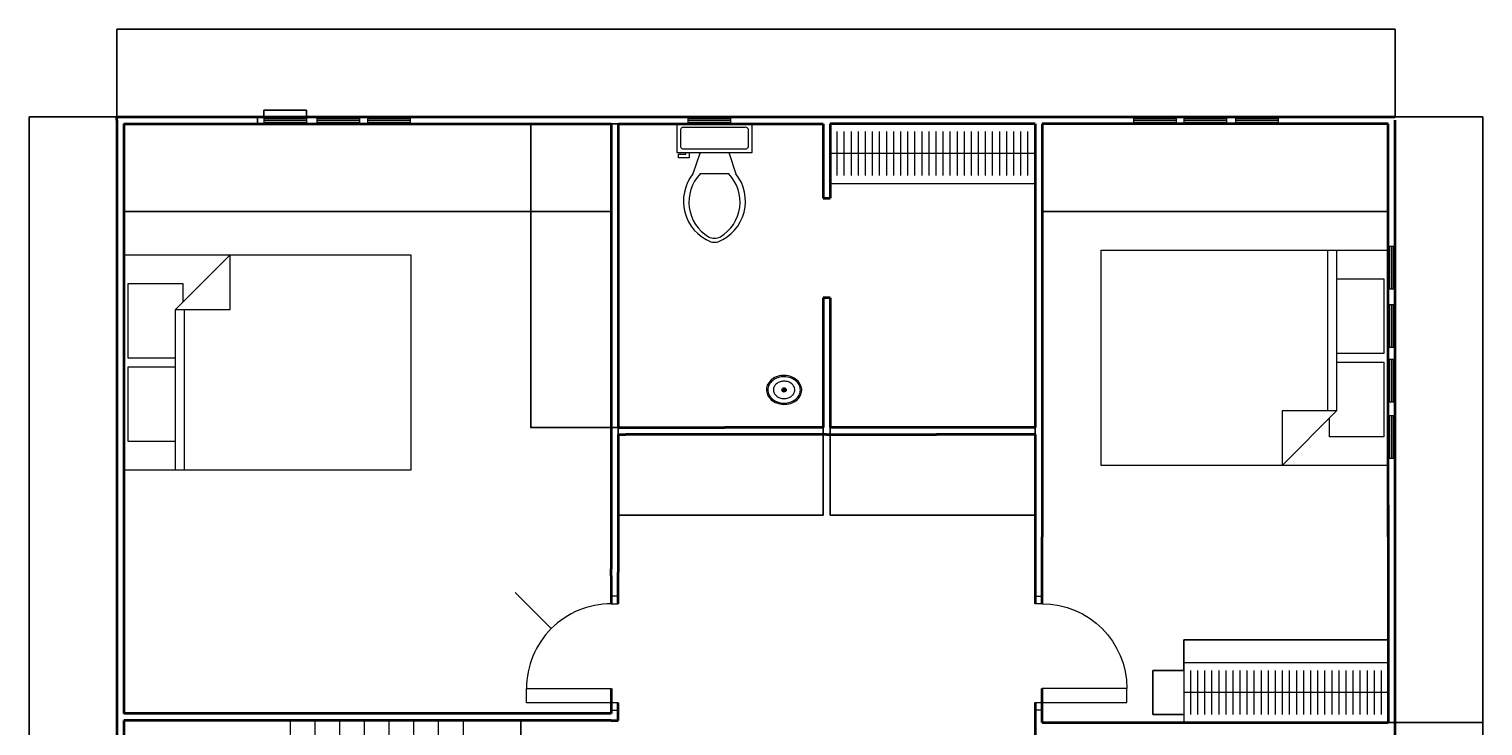
# Model space of a CAD drawing. Units: millimetres. Extents: x 1194 to 22780, y 83 to 13378.
# Tile 6 of 6: x 12489 to 22780, y 8443 to 13376. Entities that reach past the tile are written whole.
import ezdxf

# ---------------------------------------------------------------- set-up
doc = ezdxf.new("R2010")
doc.units = ezdxf.units.MM
for name, color, linetype, lineweight in [('A-ANNO-DIMS', 2, 'Continuous', 18), ('A-DOOR', 3, 'Continuous', 18), ('A-FLOR-CASE', 8, 'Continuous', 13), ('A-FLOR-FIXT', 9, 'Continuous', 18), ('A-FLOR-STRS', 7, 'Continuous', 18), ('A-FURN', 8, 'Continuous', 18), ('A-GLAZ', 4, 'Continuous', 18), ('A-WALL', 7, 'Continuous', 35)]:
    doc.layers.add(name, color=color, linetype=linetype, lineweight=lineweight)
doc.styles.get("Standard").update_dxf_attribs({"font": 'arial.ttf'})
doc.dimstyles.get("Standard").update_dxf_attribs({"dimtxt": 0.18, "dimasz": 0.18, "dimexe": 0.18, "dimexo": 0.0625, "dimgap": 0.09, "dimtad": 0, "dimtih": 1, "dimtoh": 1, "dimdec": 4, "dimzin": 0, "dimdsep": 46, "dimtxsty": 'Standard', "dimcen": 0.09, "dimadec": 0, "dimazin": 0, "dimtfac": 1, "dimtdec": 4, "dimtofl": 0, "dimtmove": 0, "dimatfit": 3, "dimfxl": 1, "dimtolj": 1, "dimtzin": 0, "dimarcsym": 0})

# ---------------------------------------------------------------- blocks, each defined once
blk = doc.blocks.new('Window - Wood Frame 36 in. Wide plan')
for p, q in [((0, 6), (0, 0)), ((0, 4.5), (36, 4.5)), ((0, 3), (36, 3)), ((0, 1.5), (36, 1.5)), ((36, 6), (36, 0))]:
    blk.add_line(p, q)
blk = doc.blocks.new('Bed - Queen')
for p, q in [((0, -80.00003000000002), (0, 0)), ((0, 0), (59.99998999999999, 0)), ((59.99998999999999, 0), (59.99998999999999, -80.00003000000002)), ((7.99999, -1.200000000000017), (28.79998, -1.200000000000017)), ((7.99999, -14.4), (7.99999, -1.200000000000017)), ((28.79998, -1.200000000000017), (28.79998, -14.4)), ((31.19999, -1.200000000000017), (51.99999000000001, -1.200000000000017)), ((31.19999, -14.4), (31.19999, -1.200000000000017)), ((51.99999000000001, -1.200000000000017), (51.99999000000001, -16.4)), ((0, -14.4), (44.79999999999999, -14.4)), ((59.99998999999999, -29.60000000000001), (44.79999999999999, -14.4)), ((44.79999999999999, -14.4), (44.79999999999999, -29.60000000000001)), ((44.79999999999999, -16.80000000000001), (0, -16.80000000000001)), ((51.99999000000001, -16.4), (46.79936, -16.4)), ((44.79999999999999, -29.60000000000001), (59.99998999999999, -29.60000000000001)), ((59.99998999999999, -80.00003000000002), (0, -80.00003000000002))]:
    blk.add_line(p, q)
blk = doc.blocks.new('Toilet - top')
for p, q in [((9.5, -6), (9.5, -2)), ((-8, -8.5), (-8, -8)), ((-7, -8), (-7, -9.5)), ((-4, -8), (-6, -14)), ((4, -8), (6, -14)), ((-10, -8.5), (-8, -8.5)), ((-10, -9.5), (-10, -8.5)), ((-7, -9.5), (-10, -9.5)), ((4, -14), (-4, -14))]:
    blk.add_line(p, q)
blk.add_lwpolyline([(10.5, -8), (10.5, 0), (-10.5, 0), (-10.5, -8)], close=True)
for points in [[(-9.5, -2), (-9.5, -6)], [(8.5, -1), (-8.5, -1)], [(-8.5, -7), (8.5, -7)]]:
    blk.add_lwpolyline(points)
for centre, radius, start, end in [((-8.625, -1.875), 0.8838834999999999, 81.86989999999999, 188.1301), ((8.625, -1.875), 0.8838834999999999, 351.8699, 98.13009999999998), ((-8.625, -6.125), 0.8838834999999999, 171.869898, 278.1301), ((8.625, -6.125), 0.8838834999999999, 261.8699, 8.130099999999993), ((3.519562435188956, -21.58049502388982), 12.16902005083646, 141.4691096810948, 247.9714346835576), ((4.199957580658807, -21.81740929088453), 11.3291791325804, 136.3677254423718, 238.946823937405), ((-3.519499936778316, -21.58047137067522), 12.16903423757823, 292.0284332733152, 38.53070636800453), ((-4.199890672038477, -21.81738596564128), 11.32918622148567, 301.0530065773863, 43.63209216694732), ((2.09660981727e-05, -27.87646475467881), 4, 245.7318247449371, 294.2681740488959), ((2.09415214183e-05, -28.99996806116075), 4, 254.8605283244437, 285.1394707718433)]:
    blk.add_arc(centre, radius, start, end)
blk = doc.blocks.new('Sink - Oval top')
for p, q in [((-1, 0), (1, 0)), ((0, 1), (0, -1))]:
    blk.add_line(p, q)
for points in [[(-12.23371880354079, 0.3941914712607968, 0.1176342565883263), (-11.46456229543957, -3.361933235489118, 0.104469279667093), (-8.878748691070427, -6.803541973650567, 0.0900157896014849), (-5.082757700676665, -9.072309807490512, 0.0819199491592185), (-0.3227280122732736, -10.01585280257211, 0.0819199491592091), (4.488169920880977, -9.380701564817912, 0.0900157896014801), (8.422342359155778, -7.36101289847943, 0.1044692796670922), (11.22435122606941, -4.093009071543406, 0.1176342565883338), (12.23371880354091, -0.3941914712607968, 0.1176342565883057), (11.46456229543992, 3.361933235488777, 0.1044692796670849), (8.878748691070427, 6.803541973650567, 0.0900157896014884), (5.082757700676324, 9.072309807490681, 0.0819199491592058), (0.3227280122732736, 10.01585280257211, 0.081919949159207), (-4.488169920880864, 9.380701564817969, 0.0900157896014802), (-8.422342359155778, 7.36101289847943, 0.1044692796670951), (-11.22435122606919, 4.093009071543633, 0.1176342565883402)], [(-11.28627986850119, 0.1590597164737346, 0.1186217001864142), (-10.51590095791209, -3.253161772358112, 0.1046781721811095), (-8.071803350560115, -6.358618019863342, 0.0895620664691738), (-4.537699193222351, -8.366971929609804, 0.0811846988912177), (-0.1289739026695997, -9.15150355811437, 0.0811846988912276), (4.300109150126218, -8.491524865184601, 0.0895620664691798), (7.889406708212618, -6.583562428127606, 0.1046781721811044), (10.42004782883111, -3.548216131892445, 0.1186217001864013), (11.28627986850119, -0.1590597164736209, 0.1186217001863945), (10.51590095791221, 3.253161772357998, 0.1046781721811069), (8.071803350560115, 6.358618019863342, 0.0895620664691756), (4.537699193222124, 8.366971929609917, 0.081184698891216), (0.1289739026695997, 9.151503558114428, 0.0811846988912142), (-4.300109150125877, 8.491524865184829, 0.0895620664691747), (-7.889406708212618, 6.583562428127606, 0.1046781721811045), (-10.42004782883111, 3.548216131892445, 0.1186217001863946)], [(-7.420452389032902, 0.0829876781601797, 0.1182825673856775), (-6.907065465214486, -2.1674649380775, 0.1046074595377274), (-5.294791470712084, -4.209988192029413, 0.0897179636260996), (-2.966599981142508, -5.528122152688069, 0.0814360825277113), (-0.0675135187855176, -6.036810076758797, 0.0814360825277218), (2.84222437824053, -5.593085960977873, 0.0897179636261315), (5.199312936802016, -4.327350491993342, 0.1046074595376878), (6.85686365682659, -2.321395784920355, 0.1182825673856714), (7.420452389033016, -0.0829876781601797, 0.1182825673856961), (6.907065465214486, 2.167464938077614, 0.1046074595377135), (5.294791470712084, 4.209988192029413, 0.0897179636261265), (2.966599981142621, 5.528122152687842, 0.0814360825277426), (0.0675135187855176, 6.036810076758797, 0.0814360825277225), (-2.842224378240644, 5.593085960977873, 0.0897179636261212), (-5.199312936802016, 4.327350491993342, 0.1046074595377049), (-6.856863656826476, 2.321395784920355, 0.1182825673856712)]]:
    blk.add_lwpolyline(points, format="xyb", close=True)
for radius in [1.5, 1]:
    blk.add_circle((0, 0), radius)
blk = doc.blocks.new('DOOR-SWING-600')
for p, q in [((-0.0004640084134735, -0.0001152583831754), (-0.0004640084134735, 599.9998847416168)), ((-0.0004640084134735, 599.9998847416168), (99.99953599158653, 599.9998847416168)), ((99.99953599158653, 599.9998847416168), (99.99953599158653, -0.0001152583831754))]:
    blk.add_line(p, q)
blk.add_arc((99.99953599158653, -0.0001152583831754), 600, 0, 90)
blk = doc.blocks.new('STAIR-DUPLEX-FLIGHT')
for p, q in [((1176.96885325314, 2725.862485348514), (1176.968853253142, -0.0001152583818111)), ((1351.817410696747, 2725.862485348514), (1351.817410696749, -0.0001152583818111)), ((1526.665968140353, 2725.862485348514), (1526.665968140356, -0.0001152583818111)), ((1701.514525583962, 2725.862485348514), (1701.514525583963, -0.0001152583818111)), ((1876.363083027568, 2725.862485348514), (1876.36308302757, -0.0001152583818111)), ((2051.211640471177, 2725.862485348514), (2051.211640471178, -0.0001152583818111)), ((2226.060197914782, 2725.862485348514), (2226.060197914785, -0.0001152583818111)), ((2400.908755358392, 2725.862485348514), (2400.908755358392, -0.0001152583818111)), ((1176.968853253141, 1562.931185045065), (0.0001000200393264, 1562.931185045065)), ((2400.908755358392, 1562.931185045066), (1176.968853253141, 1562.931185045065)), ((1186.968853253141, 1552.931185045065), (2390.908755358392, 1552.931185045065)), ((1186.968853253141, 1172.931185045065), (1186.968853253141, 1552.931185045064)), ((2390.908755358392, 1552.931185045065), (2390.908755358392, 1172.931185045064)), ((2400.908755358392, 1362.931185045066), (2400.908755358392, 1562.931185045066)), ((2400.908755358392, 1162.931185045065), (0.0001000200397812, 1162.931185045066)), ((2390.908755358392, 1172.931185045065), (1186.968853253141, 1172.931185045065))]:
    blk.add_line(p, q)
blk = doc.blocks.new('WARDROBE-RAIL-1450')
for p, q in [((50.00009064076585, 156.2053464391829), (50.00009064076585, 312.4110051556672)), ((100.0000906407658, 156.2053464391829), (100.0000906407658, 312.4110051556672)), ((150.0000906407658, 156.2053464391829), (150.0000906407658, 312.4110051556672)), ((200.0000906407659, 156.2053464391829), (200.0000906407659, 312.4110051556672)), ((250.0000906407659, 156.2053464391829), (250.0000906407659, 312.4110051556672)), ((300.0000906407659, 156.2053464391829), (300.0000906407659, 312.4110051556672)), ((350.0000906407659, 156.2053464391829), (350.0000906407659, 312.4110051556672)), ((400.0000906407658, 156.2053464391829), (400.0000906407658, 312.4110051556672)), ((450.0000906407658, 156.2053464391847), (450.0000906407658, 312.411005155669)), ((500.0000906407658, 156.2053464391847), (500.0000906407658, 312.411005155669)), ((550.0000906407658, 156.2053464391847), (550.0000906407658, 312.411005155669)), ((600.0000906407658, 156.2053464391847), (600.0000906407658, 312.411005155669)), ((650.0000906407658, 156.2053464391847), (650.0000906407658, 312.411005155669)), ((700.0000906407658, 156.2053464391847), (700.0000906407658, 312.411005155669)), ((750.0000906407658, 156.2053464391847), (750.0000906407658, 312.411005155669)), ((800.0000906407658, 156.2053464391847), (800.0000906407658, 312.411005155669)), ((850.0000906407658, 156.2053464391847), (850.0000906407658, 312.411005155669)), ((900.0000906407658, 156.2053464391847), (900.0000906407658, 312.411005155669)), ((950.0000906407658, 156.2053464391847), (950.0000906407658, 312.411005155669)), ((1000.000090640766, 156.2053464391847), (1000.000090640766, 312.411005155669)), ((1050.000090640766, 156.2053464391847), (1050.000090640766, 312.411005155669)), ((1100.000090640766, 156.2053464391847), (1100.000090640766, 312.411005155669)), ((1150.000090640766, 156.2053464391847), (1150.000090640766, 312.411005155669)), ((1200.000090640766, 156.2053464391847), (1200.000090640766, 312.411005155669)), ((1250.000090640766, 156.2053464391847), (1250.000090640766, 312.411005155669)), ((1300.000090640766, 156.2053464391847), (1300.000090640766, 312.411005155669)), ((1350.000090640766, 156.2053464391847), (1350.000090640766, 312.411005155669)), ((1400.000090640766, 156.2053464391847), (1400.000090640766, 312.411005155669)), ((1450.000090640766, 156.2053464391847), (1450.000090640766, 312.411005155669)), ((1450.000090640766, 156.2053464391847), (9.06407658476e-05, 156.2053464391847)), ((50.00009064076585, -0.0003122773014184), (50.00009064076585, 156.2053464391829)), ((100.0000906407658, -0.0003122773014184), (100.0000906407658, 156.2053464391829)), ((150.0000906407658, -0.0003122773014184), (150.0000906407658, 156.2053464391829)), ((200.0000906407659, -0.0003122773014184), (200.0000906407659, 156.2053464391829)), ((250.0000906407659, -0.0003122773014184), (250.0000906407659, 156.2053464391829)), ((300.0000906407659, -0.0003122773014184), (300.0000906407659, 156.2053464391829)), ((350.0000906407659, -0.0003122773014184), (350.0000906407659, 156.2053464391829)), ((400.0000906407658, -0.0003122773014184), (400.0000906407658, 156.2053464391829)), ((450.0000906407658, -0.0003122772995994), (450.0000906407658, 156.2053464391847)), ((500.0000906407658, -0.0003122772995994), (500.0000906407658, 156.2053464391847)), ((550.0000906407658, -0.0003122772995994), (550.0000906407658, 156.2053464391847)), ((600.0000906407658, -0.0003122772995994), (600.0000906407658, 156.2053464391847)), ((650.0000906407658, -0.0003122772995994), (650.0000906407658, 156.2053464391847)), ((700.0000906407658, -0.0003122772995994), (700.0000906407658, 156.2053464391847)), ((750.0000906407658, -0.0003122772995994), (750.0000906407658, 156.2053464391847)), ((800.0000906407658, -0.0003122772995994), (800.0000906407658, 156.2053464391847)), ((850.0000906407658, -0.0003122772995994), (850.0000906407658, 156.2053464391847)), ((900.0000906407658, -0.0003122772995994), (900.0000906407658, 156.2053464391847)), ((950.0000906407658, -0.0003122772995994), (950.0000906407658, 156.2053464391847)), ((1000.000090640766, -0.0003122772995994), (1000.000090640766, 156.2053464391847)), ((1050.000090640766, -0.0003122772995994), (1050.000090640766, 156.2053464391847)), ((1100.000090640766, -0.0003122772995994), (1100.000090640766, 156.2053464391847)), ((1150.000090640766, -0.0003122772995994), (1150.000090640766, 156.2053464391847)), ((1200.000090640766, -0.0003122772995994), (1200.000090640766, 156.2053464391847)), ((1250.000090640766, -0.0003122772995994), (1250.000090640766, 156.2053464391847)), ((1300.000090640766, -0.0003122772995994), (1300.000090640766, 156.2053464391847)), ((1350.000090640766, -0.0003122772995994), (1350.000090640766, 156.2053464391847)), ((1400.000090640766, -0.0003122772995994), (1400.000090640766, 156.2053464391847))]:
    blk.add_line(p, q)
blk = doc.blocks.new('*D17')
at = {"layer": 'A-ANNO-DIMS', "color": 0, "lineweight": -2, "transparency": 16777216}
for p, q in [((14151.05908825639, 12755.83638474161), (14151.05908825639, 12801.24910150435)), ((14151.23908825639, 12801.06910150435), (14300.85484945277, 12801.06910150435)), ((14452.84720000795, 12801.06910150435), (14303.23143881157, 12801.06910150435)), ((14453.02720000795, 12755.83638474161), (14453.02720000795, 12801.24910150435))]:
    blk.add_line(p, q, dxfattribs=at)
at = {"layer": 'A-ANNO-DIMS', "color": 0, "transparency": 16777216}
for points in [[(14151.23908825639, 12801.09910150435), (14151.23908825639, 12801.03910150435), (14151.05908825639, 12801.06910150435)], [(14452.84720000795, 12801.09910150435), (14452.84720000795, 12801.03910150435), (14453.02720000795, 12801.06910150435)]]:
    blk.add_solid(points, dxfattribs=at)
at = {"layer": 'Defpoints', "color": 0, "transparency": 16777216}
for p in [(14453.02720000795, 12801.06910150435), (14151.05908825639, 12755.77388474161), (14453.02720000795, 12755.77388474161)]:
    blk.add_point(p, dxfattribs=at)
at = {"layer": 'A-ANNO-DIMS', "color": 0, "transparency": 16777216, "insert": (14302.04314413217, 12801.06910150435), "char_height": 0.18, "attachment_point": 5}
blk.add_mtext('\\A1;WINDOW 302 TYP.', dxfattribs=at)
blk = doc.blocks.new('*D18')
at = {"layer": 'A-ANNO-DIMS', "color": 0, "lineweight": -2, "transparency": 16777216}
for p, q in [((14150.99658825639, 12755.77388474162), (14105.58387149367, 12755.77388474162)), ((14150.99658825639, 12705.44586611636), (14105.58387149367, 12705.44586611636)), ((14105.76387149367, 12755.59388474162), (14105.76387149367, 12730.79177856678)), ((14105.76387149367, 12705.62586611636), (14105.76387149367, 12730.4279722912))]:
    blk.add_line(p, q, dxfattribs=at)
at = {"layer": 'A-ANNO-DIMS', "color": 0, "transparency": 16777216}
for points in [[(14105.73387149367, 12755.59388474162), (14105.79387149367, 12755.59388474162), (14105.76387149367, 12755.77388474162)], [(14105.73387149367, 12705.62586611636), (14105.79387149367, 12705.62586611636), (14105.76387149367, 12705.44586611636)]]:
    blk.add_solid(points, dxfattribs=at)
at = {"layer": 'Defpoints', "color": 0, "transparency": 16777216}
for p in [(14105.76387149367, 12755.77388474162), (14151.0590882564, 12755.77388474162), (14151.0590882564, 12705.44586611636)]:
    blk.add_point(p, dxfattribs=at)
at = {"layer": 'A-ANNO-DIMS', "color": 0, "transparency": 16777216, "insert": (14105.76387149367, 12730.60987542898), "char_height": 0.18, "attachment_point": 5}
blk.add_mtext('\\A1;50 TYP.', dxfattribs=at)
blk = doc.blocks.new('*D29')
at = {"layer": 'A-ANNO-DIMS', "color": 0, "lineweight": -2, "transparency": 16777216}
for p, q in [((20661.40509064076, 8835.72550515567), (20661.40509064076, 9053.34300515567)), ((20661.58509064076, 9053.16300515567), (21384.88577276901, 9053.16300515567)), ((22111.22509064077, 9053.16300515567), (21387.92440851252, 9053.16300515567)), ((22111.40509064076, 8835.72550515567), (22111.40509064076, 9053.34300515567))]:
    blk.add_line(p, q, dxfattribs=at)
at = {"layer": 'A-ANNO-DIMS', "color": 0, "transparency": 16777216}
for points in [[(20661.58509064076, 9053.193005155668), (20661.58509064076, 9053.13300515567), (20661.40509064076, 9053.16300515567)], [(22111.22509064077, 9053.193005155668), (22111.22509064077, 9053.13300515567), (22111.40509064076, 9053.16300515567)]]:
    blk.add_solid(points, dxfattribs=at)
at = {"layer": 'Defpoints', "color": 0, "transparency": 16777216}
for p in [(22111.40509064076, 9053.16300515567), (20661.40509064076, 8835.66300515567), (22111.40509064076, 8835.66300515567)]:
    blk.add_point(p, dxfattribs=at)
at = {"layer": 'A-ANNO-DIMS', "color": 0, "transparency": 16777216, "insert": (21386.40509064077, 9053.16300515567), "char_height": 0.18, "attachment_point": 5}
blk.add_mtext('\\A1;CLOSET RAIL 1450 TYP.', dxfattribs=at)
blk = doc.blocks.new('*D30')
at = {"layer": 'A-ANNO-DIMS', "color": 0, "lineweight": -2, "transparency": 16777216}
for p, q in [((20661.34259064077, 8835.663005155673), (20443.72509064078, 8835.663005155671)), ((20443.90509064078, 8835.483005155671), (20443.90509064078, 8679.639310968516)), ((20443.90509064078, 8523.431687722701), (20443.90509064078, 8679.275381909854)), ((20661.34259064077, 8523.251687722703), (20443.72509064078, 8523.251687722703))]:
    blk.add_line(p, q, dxfattribs=at)
at = {"layer": 'A-ANNO-DIMS', "color": 0, "transparency": 16777216}
for points in [[(20443.87509064078, 8835.483005155671), (20443.93509064078, 8835.483005155671), (20443.90509064078, 8835.663005155671)], [(20443.87509064078, 8523.431687722701), (20443.93509064078, 8523.431687722701), (20443.90509064078, 8523.251687722703)]]:
    blk.add_solid(points, dxfattribs=at)
at = {"layer": 'Defpoints', "color": 0, "transparency": 16777216}
for p in [(20443.90509064078, 8835.663005155671), (20661.40509064077, 8835.663005155673), (20661.40509064077, 8523.251687722703)]:
    blk.add_point(p, dxfattribs=at)
at = {"layer": 'A-ANNO-DIMS', "color": 0, "transparency": 16777216, "insert": (20443.90509064078, 8679.457346439178), "char_height": 0.18, "attachment_point": 5}
blk.add_mtext('\\A1;312 TYP.', dxfattribs=at)
blk = doc.blocks.new('*D39')
at = {"layer": 'A-ANNO-DIMS', "color": 0, "lineweight": -2, "transparency": 16777216}
for p, q in [((15560.17780421591, 8481.63648534852), (15969.17469430695, 8481.63648534852)), ((15968.99469430695, 8481.45648534852), (15968.99469430695, 7118.888254622152)), ((15968.99469430695, 5755.953884741622), (15968.99469430695, 7118.522115467991)), ((15560.17780421591, 5755.773884741622), (15969.17469430695, 5755.773884741622))]:
    blk.add_line(p, q, dxfattribs=at)
at = {"layer": 'A-ANNO-DIMS', "color": 0, "transparency": 16777216}
for points in [[(15968.96469430695, 8481.45648534852), (15969.02469430695, 8481.45648534852), (15968.99469430695, 8481.63648534852)], [(15968.96469430695, 5755.953884741622), (15969.02469430695, 5755.953884741622), (15968.99469430695, 5755.773884741622)]]:
    blk.add_solid(points, dxfattribs=at)
at = {"layer": 'Defpoints', "color": 0, "transparency": 16777216}
for p in [(15560.11530421591, 8481.63648534852), (15968.99469430695, 8481.63648534852), (15560.11530421591, 5755.773884741622)]:
    blk.add_point(p, dxfattribs=at)
at = {"layer": 'A-ANNO-DIMS', "color": 0, "transparency": 16777216, "insert": (15968.99469430695, 7118.705185045065), "char_height": 0.18, "attachment_point": 5}
blk.add_mtext('\\A1;STAIR 2726 TYP.', dxfattribs=at)
blk = doc.blocks.new('*D72')
at = {"layer": 'A-ANNO-DIMS', "color": 0, "lineweight": -2, "transparency": 16777216}
for p, q in [((13109.206649, 12755.836385), (13109.206649, 13375.953885)), ((13109.386649, 13375.773885), (17633.84818378854, 13375.773885)), ((22159.026649, 13375.773885), (17634.56511421146, 13375.773885)), ((22159.206649, 12755.836385), (22159.206649, 13375.953885))]:
    blk.add_line(p, q, dxfattribs=at)
at = {"layer": 'A-ANNO-DIMS', "color": 0, "transparency": 16777216}
for points in [[(13109.386649, 13375.803885), (13109.386649, 13375.743885), (13109.206649, 13375.773885)], [(22159.026649, 13375.803885), (22159.026649, 13375.743885), (22159.206649, 13375.773885)]]:
    blk.add_solid(points, dxfattribs=at)
at = {"layer": 'Defpoints', "color": 0, "transparency": 16777216}
for p in [(22159.206649, 13375.773885), (13109.206649, 12755.773885), (22159.206649, 12755.773885)]:
    blk.add_point(p, dxfattribs=at)
at = {"layer": 'A-ANNO-DIMS', "color": 0, "transparency": 16777216, "insert": (17634.206649, 13375.773885), "char_height": 0.18, "attachment_point": 5}
blk.add_mtext('\\A1;9050', dxfattribs=at)
blk = doc.blocks.new('*D73')
at = {"layer": 'A-ANNO-DIMS', "color": 0, "lineweight": -2, "transparency": 16777216}
for p, q in [((13109.144149, 12755.77388500001), (12488.69863000001, 12755.77388500001)), ((12488.87863000001, 12755.593885), (12488.87863000001, 6755.977501137794)), ((12488.87863000001, 755.9973109999999), (12488.87863000001, 6755.613694862214)), ((13109.144149, 755.8173110000002), (12488.69863000001, 755.817311))]:
    blk.add_line(p, q, dxfattribs=at)
at = {"layer": 'A-ANNO-DIMS', "color": 0, "transparency": 16777216}
for points in [[(12488.84863000001, 12755.593885), (12488.90863000001, 12755.593885), (12488.87863000001, 12755.77388500001)], [(12488.84863000001, 755.9973109999999), (12488.90863000001, 755.9973109999999), (12488.87863000001, 755.817311)]]:
    blk.add_solid(points, dxfattribs=at)
at = {"layer": 'Defpoints', "color": 0, "transparency": 16777216}
for p in [(12488.87863000001, 12755.77388500001), (13109.206649, 12755.77388500001), (13109.206649, 755.8173110000002)]:
    blk.add_point(p, dxfattribs=at)
at = {"layer": 'A-ANNO-DIMS', "color": 0, "transparency": 16777216, "insert": (12488.87863000001, 6755.795597999997), "char_height": 0.18, "attachment_point": 5}
blk.add_mtext('\\A1;12000', dxfattribs=at)
blk = doc.blocks.new('*D77')
at = {"layer": 'A-ANNO-DIMS', "color": 0, "lineweight": -2, "transparency": 16777216}
for p, q in [((22109.26914900001, 8468.273885000004), (22779.38664900001, 8468.273885000004)), ((22779.20664900001, 8468.093885000006), (22779.20664900002, 7112.205788137794)), ((22779.20664900002, 5755.953885000002), (22779.20664900002, 7111.841981862214)), ((22109.26914900001, 5755.773885000001), (22779.38664900001, 5755.773885000002))]:
    blk.add_line(p, q, dxfattribs=at)
at = {"layer": 'A-ANNO-DIMS', "color": 0, "transparency": 16777216}
for points in [[(22779.17664900001, 8468.093885000006), (22779.23664900001, 8468.093885000006), (22779.20664900001, 8468.273885000004)], [(22779.17664900002, 5755.953885000002), (22779.23664900002, 5755.953885000002), (22779.20664900002, 5755.773885000002)]]:
    blk.add_solid(points, dxfattribs=at)
at = {"layer": 'Defpoints', "color": 0, "transparency": 16777216}
for p in [(22109.20664900001, 8468.273885000004), (22779.20664900001, 8468.273885000004), (22109.20664900001, 5755.773885000001)]:
    blk.add_point(p, dxfattribs=at)
at = {"layer": 'A-ANNO-DIMS', "color": 0, "transparency": 16777216, "insert": (22779.20664900001, 7112.023884999995), "char_height": 0.18, "attachment_point": 5}
blk.add_mtext('\\A1;2712.5', dxfattribs=at)
blk = doc.blocks.new('*D78')
at = {"layer": 'A-ANNO-DIMS', "color": 0, "lineweight": -2, "transparency": 16777216}
for p, q in [((22159.26914900001, 12755.77388500001), (22779.38664900001, 12755.77388500001)), ((22779.20664900002, 12755.593885), (22779.20664900002, 10612.20578813779)), ((22779.20664900002, 8468.453885000004), (22779.20664900002, 10611.84198186222)), ((22109.26914900001, 8468.273885000004), (22779.38664900001, 8468.273885000004))]:
    blk.add_line(p, q, dxfattribs=at)
at = {"layer": 'A-ANNO-DIMS', "color": 0, "transparency": 16777216}
for points in [[(22779.17664900002, 12755.593885), (22779.23664900002, 12755.593885), (22779.20664900002, 12755.77388500001)], [(22779.17664900002, 8468.453885000004), (22779.23664900002, 8468.453885000004), (22779.20664900002, 8468.273885000004)]]:
    blk.add_solid(points, dxfattribs=at)
at = {"layer": 'Defpoints', "color": 0, "transparency": 16777216}
for p in [(22159.20664900001, 12755.77388500001), (22779.20664900002, 12755.77388500001), (22109.20664900001, 8468.273885000004)]:
    blk.add_point(p, dxfattribs=at)
at = {"layer": 'A-ANNO-DIMS', "color": 0, "transparency": 16777216, "insert": (22779.20664900002, 10612.02388499999), "char_height": 0.18, "attachment_point": 5}
blk.add_mtext('\\A1;4287.5', dxfattribs=at)
blk = doc.blocks.new('*D79')
at = {"layer": 'A-ANNO-DIMS', "color": 0, "lineweight": -2, "transparency": 16777216}
for p, q in [((16659.206649, 10555.711385), (16659.206649, 9935.593885)), ((18109.206649, 10555.711385), (18109.206649, 9935.593885)), ((16659.386649, 9935.773885), (17383.85665582128, 9935.773885)), ((18109.026649, 9935.773885), (17384.55664217872, 9935.773885))]:
    blk.add_line(p, q, dxfattribs=at)
at = {"layer": 'A-ANNO-DIMS', "color": 0, "transparency": 16777216}
for points in [[(16659.386649, 9935.803885000001), (16659.386649, 9935.743885), (16659.206649, 9935.773885)], [(18109.026649, 9935.803885000001), (18109.026649, 9935.743885), (18109.206649, 9935.773885)]]:
    blk.add_solid(points, dxfattribs=at)
at = {"layer": 'Defpoints', "color": 0, "transparency": 16777216}
for p in [(16659.206649, 10555.773885), (18109.206649, 10555.773885), (16659.206649, 9935.773885)]:
    blk.add_point(p, dxfattribs=at)
at = {"layer": 'A-ANNO-DIMS', "color": 0, "transparency": 16777216, "insert": (17384.206649, 9935.773885), "char_height": 0.18, "attachment_point": 5}
blk.add_mtext('\\A1;1450', dxfattribs=at)
blk = doc.blocks.new('*D80')
at = {"layer": 'A-ANNO-DIMS', "color": 0, "lineweight": -2, "transparency": 16777216}
for p, q in [((18159.206649, 10555.711385), (18159.20664899999, 9935.593885000006)), ((19609.206649, 10555.711385), (19609.20664899999, 9935.593884999995)), ((18159.38664899999, 9935.773885000006), (18883.85665582127, 9935.773885)), ((19609.02664899999, 9935.773884999997), (18884.55664217871, 9935.773885))]:
    blk.add_line(p, q, dxfattribs=at)
at = {"layer": 'A-ANNO-DIMS', "color": 0, "transparency": 16777216}
for points in [[(18159.38664899999, 9935.803885000007), (18159.38664899999, 9935.743885000005), (18159.20664899999, 9935.773885000006)], [(19609.02664899999, 9935.803884999996), (19609.02664899999, 9935.743884999994), (19609.20664899999, 9935.773884999997)]]:
    blk.add_solid(points, dxfattribs=at)
at = {"layer": 'Defpoints', "color": 0, "transparency": 16777216}
for p in [(18159.206649, 10555.773885), (19609.206649, 10555.773885), (18159.20664899999, 9935.773885000006)]:
    blk.add_point(p, dxfattribs=at)
at = {"layer": 'A-ANNO-DIMS', "color": 0, "transparency": 16777216, "insert": (18884.20664899999, 9935.773885), "char_height": 0.18, "attachment_point": 5}
blk.add_mtext('\\A1;1450', dxfattribs=at)
blk = doc.blocks.new('*D81')
at = {"layer": 'A-ANNO-DIMS', "color": 0, "lineweight": -2, "transparency": 16777216}
for p, q in [((16659.144149, 12705.77388500001), (16039.02664900001, 12705.77388500001)), ((16039.20664900001, 12705.59388500001), (16039.20664900001, 11630.95578813779)), ((16039.20664900001, 10555.953885), (16039.20664900001, 11630.59198186221)), ((16659.144149, 10555.773885), (16039.02664900001, 10555.773885))]:
    blk.add_line(p, q, dxfattribs=at)
at = {"layer": 'A-ANNO-DIMS', "color": 0, "transparency": 16777216}
for points in [[(16039.17664900001, 12705.59388500001), (16039.23664900001, 12705.59388500001), (16039.20664900001, 12705.77388500001)], [(16039.17664900001, 10555.953885), (16039.23664900001, 10555.953885), (16039.20664900001, 10555.773885)]]:
    blk.add_solid(points, dxfattribs=at)
at = {"layer": 'Defpoints', "color": 0, "transparency": 16777216}
for p in [(16039.20664900001, 12705.77388500001), (16659.206649, 12705.77388500001), (16659.206649, 10555.773885)]:
    blk.add_point(p, dxfattribs=at)
at = {"layer": 'A-ANNO-DIMS', "color": 0, "transparency": 16777216, "insert": (16039.20664900001, 11630.77388499999), "char_height": 0.18, "attachment_point": 5}
blk.add_mtext('\\A1;2150', dxfattribs=at)
blk = doc.blocks.new('*D82')
at = {"layer": 'A-ANNO-DIMS', "color": 0, "lineweight": -2, "transparency": 16777216}
for p, q in [((13159.206649, 12705.711385), (13159.206649, 12085.593885)), ((16609.206649, 12705.711385), (16609.206649, 12085.593885)), ((13159.386649, 12085.773885), (14883.84824518008, 12085.773885)), ((16609.026649, 12085.773885), (14884.56505281992, 12085.773885))]:
    blk.add_line(p, q, dxfattribs=at)
at = {"layer": 'A-ANNO-DIMS', "color": 0, "transparency": 16777216}
for points in [[(13159.386649, 12085.803885), (13159.386649, 12085.743885), (13159.206649, 12085.773885)], [(16609.026649, 12085.803885), (16609.026649, 12085.743885), (16609.206649, 12085.773885)]]:
    blk.add_solid(points, dxfattribs=at)
at = {"layer": 'Defpoints', "color": 0, "transparency": 16777216}
for p in [(13159.206649, 12705.773885), (16609.206649, 12705.773885), (13159.206649, 12085.773885)]:
    blk.add_point(p, dxfattribs=at)
at = {"layer": 'A-ANNO-DIMS', "color": 0, "transparency": 16777216, "insert": (14884.206649, 12085.773885), "char_height": 0.18, "attachment_point": 5}
blk.add_mtext('\\A1;3450', dxfattribs=at)
blk = doc.blocks.new('*D83')
at = {"layer": 'A-ANNO-DIMS', "color": 0, "lineweight": -2, "transparency": 16777216}
for p, q in [((19659.206649, 12705.711385), (19659.206649, 12085.593885)), ((22109.206649, 12705.711385), (22109.206649, 12085.593885)), ((19659.386649, 12085.773885), (20883.846649, 12085.773885)), ((22109.026649, 12085.773885), (20884.566649, 12085.773885))]:
    blk.add_line(p, q, dxfattribs=at)
at = {"layer": 'A-ANNO-DIMS', "color": 0, "transparency": 16777216}
for points in [[(19659.386649, 12085.803885), (19659.386649, 12085.743885), (19659.206649, 12085.773885)], [(22109.026649, 12085.803885), (22109.026649, 12085.743885), (22109.206649, 12085.773885)]]:
    blk.add_solid(points, dxfattribs=at)
at = {"layer": 'Defpoints', "color": 0, "transparency": 16777216}
for p in [(19659.206649, 12705.773885), (22109.206649, 12705.773885), (19659.206649, 12085.773885)]:
    blk.add_point(p, dxfattribs=at)
at = {"layer": 'A-ANNO-DIMS', "color": 0, "transparency": 16777216, "insert": (20884.206649, 12085.773885), "char_height": 0.18, "attachment_point": 5}
blk.add_mtext('\\A1;2450', dxfattribs=at)
blk = doc.blocks.new('*D93')
at = {"layer": 'A-ANNO-DIMS', "color": 0, "lineweight": -2, "transparency": 16777216}
for p, q in [((15930.20484437298, 9386.630684827021), (15930.38484437298, 9386.630684827021)), ((15930.38484437298, 9386.630684827021), (16184.81574191169, 9132.199258352914)), ((16609.116649, 8707.807469000005), (16609.296649, 8707.807469000005)), ((16609.206649, 8707.717469000005), (16609.206649, 8707.897469000003))]:
    blk.add_line(p, q, dxfattribs=at)
at = {"layer": 'A-ANNO-DIMS', "color": 0, "transparency": 16777216}
blk.add_solid([(16184.83695513717, 9132.220471534298), (16184.7945286862, 9132.178045171528), (16184.943021, 9132.071979)], dxfattribs=at)
at = {"layer": 'Defpoints', "color": 0, "transparency": 16777216}
for p in [(16184.943021, 9132.071979), (16609.206649, 8707.807469000005)]:
    blk.add_point(p, dxfattribs=at)
at = {"layer": 'A-ANNO-DIMS', "color": 0, "transparency": 16777216, "insert": (15929.63666565538, 9386.630684827021), "char_height": 0.18, "attachment_point": 5}
blk.add_mtext('\\A1;8X R600', dxfattribs=at)

msp = doc.modelspace()

# ---------------------------------------------------------------- linework, layer by layer
at = {"layer": 'A-DOOR'}
for p, q in [((16659.20664887754, 9361.492341907959), (16609.20664887754, 9361.492341907959)), ((16609.20664887754, 9307.807469076275), (16659.20664887754, 9307.807469076275)), ((19609.20664887754, 9362.117260640807), (19659.20664887754, 9362.117260640807)), ((19609.20664887754, 9308.432387809125), (19609.20664887754, 9362.117260640807)), ((19609.20664887754, 9362.117260640807), (19659.20664887754, 9362.117260640807)), ((19659.20664887754, 9308.432387809125), (19609.20664887754, 9308.432387809125)), ((19659.20664887754, 9362.117260640807), (19659.20664887754, 9308.432387809125)), ((16609.20664887754, 8554.12259624459), (16609.20664887754, 8707.807469076275)), ((19659.20664887754, 8554.747514977442), (19659.20664887754, 8708.432387809124)), ((16659.20664887754, 8607.807469076275), (16609.20664887754, 8607.807469076275)), ((16609.20664887754, 8554.12259624459), (16659.20664887754, 8554.12259624459)), ((16659.20664887754, 8554.12259624459), (16659.20664887754, 8607.807469076275)), ((19609.20664887754, 8554.747514977442), (19609.20664887754, 8608.432387809124)), ((19609.20664887754, 8608.432387809124), (19659.20664887754, 8608.432387809124)), ((19659.20664887754, 8554.747514977442), (19609.20664887754, 8554.747514977442)), ((19659.20664887754, 8554.747514977442), (19609.20664887754, 8554.747514977442))]:
    msp.add_line(p, q, dxfattribs=at)
at = {"layer": 'A-FLOR-CASE'}
for p, q in [((19609.20664887754, 12283.40696134648), (19609.20664887754, 12705.77388474162)), ((19609.20664887754, 12338.38476432756), (19609.20664887754, 12494.59042304405)), ((18159.20664887754, 12283.40696134648), (19609.20664887754, 12283.40696134648)), ((20661.40509064076, 8890.640808136748), (20661.40509064076, 8468.273884741619)), ((22111.40509064076, 8890.640808136754), (20661.40509064076, 8890.640808136754)), ((22111.40509064076, 8468.273884741619), (22111.40509064076, 8890.640808136754)), ((20661.40509064076, 8468.273884741619), (22111.40509064076, 8468.273884741619))]:
    msp.add_line(p, q, dxfattribs=at)
at = {"layer": 'A-WALL'}
for p, q in [((13109.20664887754, 12730.77388474161), (13109.20664887754, 12755.77388474162)), ((13109.20664887754, 12755.77388474162), (13134.20664887754, 12755.77388474161)), ((13109.20664887754, 12730.77388474161), (13109.20664887755, 2157.764322747982)), ((13134.20664887754, 12755.77388474161), (22159.20664887755, 12755.77388474161)), ((13159.20664887754, 12705.77388474162), (13159.20664887754, 9555.773884741615)), ((13159.20664887754, 12705.77388474162), (16609.20664887754, 12705.77388474162)), ((16609.20664887754, 12705.77388474162), (16609.20664887754, 9555.773884741615)), ((16659.20664887754, 12705.77388474162), (16659.20664887754, 10555.77388474161)), ((16659.20664887754, 12705.77388474162), (18109.20664887754, 12705.77388474162)), ((18109.20664887754, 12705.77388474161), (18109.20664887754, 12179.1905268851)), ((18159.20664887754, 12705.77388474161), (18159.20664887754, 12179.1905268851)), ((19609.20664887754, 12705.77388474162), (18159.20664887754, 12705.77388474162)), ((19609.20664887754, 12705.77388474162), (19609.20664887754, 10555.77388474161)), ((19659.20664887754, 12705.77388474162), (19659.20664887754, 10055.77388474161)), ((22109.20664887755, 12705.77388474162), (19659.20664887754, 12705.77388474162)), ((22109.20664887755, 10055.77388474161), (22109.20664887755, 12705.77388474162)), ((22159.20664887755, 1052.812771575728), (22159.20664887755, 12730.77388474161)), ((18109.20664887754, 12179.1905268851), (18159.20664887754, 12179.1905268851)), ((18159.20664887754, 11473.15829364757), (18109.20664887754, 11473.15829364757)), ((18109.20664887754, 11473.15829364756), (18109.20664887754, 10555.77388474161)), ((18159.20664887754, 11473.15829364757), (18159.20664887754, 10555.77388474162)), ((16659.20664887754, 10555.77388474161), (17412.89152170923, 10555.77388474161)), ((16659.20664887754, 10505.77388474162), (16659.20664887754, 9530.773884741619)), ((16659.20664887754, 10505.77388474162), (16712.89152170923, 10505.77388474162)), ((17412.89152170923, 10505.77388474162), (16712.89152170923, 10505.77388474162)), ((18109.20664887754, 10555.77388474161), (17412.89152170923, 10555.77388474161)), ((18134.20664887754, 10505.77388474162), (17412.89152170923, 10505.77388474162)), ((18134.20664887754, 10505.77388474162), (18912.83651934459, 10505.77388474162)), ((18912.8365193446, 10555.77388474161), (18159.20664887754, 10555.77388474162)), ((19609.20664887754, 10555.77388474161), (18912.8365193446, 10555.77388474161)), ((19609.20664887754, 10505.77388474162), (18912.83651934459, 10505.77388474162)), ((19609.20664887754, 10505.77388474162), (19609.20664887754, 10030.77388474161)), ((19609.20664887754, 10030.77388474161), (19609.20664887754, 9731.201065029272)), ((19659.20664887754, 10055.77388474161), (19659.20664887754, 9781.201065029272)), ((22109.20664887755, 9781.201065029272), (22109.20664887755, 10055.77388474161)), ((22109.20664887755, 10005.77388474161), (22109.20664887755, 8468.273884741619)), ((19659.20664887754, 9731.201065029272), (19659.20664887754, 9781.201065029272)), ((19609.20664887754, 9731.201065029272), (19609.20664887754, 9308.432387809125)), ((19659.20664887754, 9308.432387809125), (19659.20664887754, 9731.201065029272)), ((13159.20664887754, 9555.773884741615), (13159.20664887754, 9505.773884741619)), ((13159.20664887754, 9505.773884741619), (13159.20664887754, 8531.636485348512)), ((16609.20664887754, 9505.773884741615), (16609.20664887754, 9555.773884741615)), ((16609.20664887754, 9505.773884741615), (16609.20664887754, 9307.807469076275)), ((16659.20664887754, 9307.807469076275), (16659.20664887754, 9530.773884741619)), ((16609.20664887753, 8707.807469076275), (16609.20664887752, 8531.636485348514)), ((19659.20664887754, 8468.273884741619), (19659.20664887754, 8708.432387809124)), ((16659.20664887754, 8481.636485348516), (16659.20664887754, 8607.807469076275)), ((19609.20664887754, 8608.432387809124), (19609.20664887754, 8142.85298843845)), ((16609.20664887754, 8531.636485348514), (13159.20664887754, 8531.636485348514)), ((16609.20664887754, 8481.636485348516), (13159.20664887754, 8481.636485348516)), ((13159.20664887754, 8481.636485348514), (13159.20664887754, 5755.773884741616)), ((16609.20664887754, 8481.636485348516), (16659.20664887754, 8481.636485348516)), ((19659.20664887754, 8468.273884741619), (22109.20664887755, 8468.273884741619))]:
    msp.add_line(p, q, dxfattribs=at)

# ---------------------------------------------------------------- block references
at = {"layer": 'A-DOOR', "rotation": 89.99999999999984}
msp.add_blockref('DOOR-SWING-600', (16609.20653361915, 8607.807933084689), dxfattribs=at)
at = {"layer": 'A-DOOR', "extrusion": (0, 0, -1), "zscale": -1, "rotation": 90.00000000000011}
msp.add_blockref('DOOR-SWING-600', (-19659.20676413592, 8608.432851817537), dxfattribs=at)
at = {"layer": 'A-FLOR-CASE'}
for p in [(18159.2065582368, 12338.38507660486), (20661.405, 8523.252)]:
    msp.add_blockref('WARDROBE-RAIL-1450', p, dxfattribs=at)
at = {"layer": 'A-FLOR-FIXT'}
for name, p, xscale, yscale, zscale in [('Toilet - top', (17339.94810248864, 12705.77388474162), 25.4, 25.4, 25.4), ('Sink - Oval top', (17832.94434762888, 10821.79048380677), 10.19841034025665, 10.19841034025665, 10.19841034025665)]:
    msp.add_blockref(name, p, dxfattribs=dict(at, xscale=xscale, yscale=yscale, zscale=zscale))
at = {"layer": 'A-FLOR-STRS'}
msp.add_blockref('STAIR-DUPLEX-FLIGHT', (13159.20654885751, 5755.774000000002), dxfattribs=at)
at = {"layer": 'A-FURN', "xscale": 25.4, "yscale": 25.4, "zscale": 25.4}
for p, rotation in [((13159.20664887754, 10253.50724226593), 90), ((22109.20664887755, 11811.30884824128), 270)]:
    msp.add_blockref('Bed - Queen', p, dxfattribs=dict(at, rotation=rotation))
at = {"layer": 'A-GLAZ', "xscale": 8.388003104210137, "yscale": 8.388003104210137, "zscale": 8.388003104210137}
for p in [(14151.05908825639, 12705.44586611635), (14526.04983173877, 12705.44586611635), (14884.20664887754, 12705.44586611635), (17152.16386489545, 12705.44586611635), (20305.84568429106, 12705.44586611635), (20663.38105838663, 12705.44586611635), (21028.86968564077, 12705.44586611635)]:
    msp.add_blockref('Window - Wood Frame 36 in. Wide plan', p, dxfattribs=at)
at = {"layer": 'A-GLAZ', "xscale": 8.388003104210137, "yscale": 8.388003104210137, "zscale": 8.388003104210137, "rotation": 90}
for p in [(22159.20664887755, 11536.60816181757), (22159.20664887755, 11124.87239179706), (22159.20664887755, 10736.88338841312), (22159.20664887755, 10338.16018782898)]:
    msp.add_blockref('Window - Wood Frame 36 in. Wide plan', p, dxfattribs=at)

# ---------------------------------------------------------------- dimensions: what is measured, and where the dimension line sits
at = {"layer": 'A-ANNO-DIMS'}
dim = msp.add_linear_dim(base=(22159.206649, 13375.773885), p1=(13109.206649, 12755.773885), p2=(22159.206649, 12755.773885), dimstyle='Standard', override={"dimdec": 0, "dimlfac": 1, "dimrnd": 0, "dimzin": 0, "dimdsep": 46, "dimlunit": 2}, dxfattribs=at)
dim.commit()
dim.dimension.update_dxf_attribs({"geometry": '*D72', "text_midpoint": (17634.206649, 13375.773885)})
for base, p1, p2, text, picture, middle in [((14453.02720000795, 12801.06910150435), (14151.05908825639, 12755.77388474161), (14453.02720000795, 12755.77388474161), 'WINDOW <> TYP.', '*D17', (14302.04314413217, 12801.06910150435)), ((22111.40509064076, 9053.16300515567), (20661.40509064076, 8835.66300515567), (22111.40509064076, 8835.66300515567), 'CLOSET RAIL <> TYP.', '*D29', (21386.40509064077, 9053.16300515567))]:
    dim = msp.add_linear_dim(base=base, p1=p1, p2=p2, text=text, dimstyle='Standard', override={"dimdec": 0, "dimlfac": 1, "dimrnd": 0, "dimzin": 0, "dimdsep": 46, "dimlunit": 2}, dxfattribs=at)
    dim.commit()
    dim.dimension.update_dxf_attribs({"geometry": picture, "text_midpoint": middle})
for base, p1, p2, angle, override, picture, middle in [((12488.87863000001, 12755.77388500001), (13109.206649, 755.817311), (13109.206649, 12755.773885), 90, {"dimdec": 0, "dimlfac": 1, "dimrnd": 0, "dimzin": 0, "dimdsep": 46, "dimlunit": 2}, '*D73', (12488.87863000001, 6755.795597999997)), ((13159.206649, 12085.773885), (16609.206649, 12705.773885), (13159.206649, 12705.773885), 180, {"dimdec": 0, "dimlfac": 1, "dimrnd": 0, "dimzin": 0, "dimdsep": 46, "dimlunit": 2}, '*D82', (14884.206649, 12085.773885)), ((16039.20664900001, 12705.77388500001), (16659.206649, 10555.773885), (16659.206649, 12705.773885), 90, {"dimdec": 0, "dimlfac": 1, "dimrnd": 0, "dimzin": 0, "dimdsep": 46, "dimlunit": 2}, '*D81', (16039.20664900001, 11630.77388499999)), ((19659.206649, 12085.773885), (22109.206649, 12705.773885), (19659.206649, 12705.773885), 180, {"dimdec": 0, "dimlfac": 1, "dimrnd": 0, "dimzin": 0, "dimdsep": 46, "dimlunit": 2}, '*D83', (20884.206649, 12085.773885)), ((22779.20664900002, 12755.77388500001), (22109.206649, 8468.273885), (22159.206649, 12755.773885), 90, {"dimdec": 1, "dimlfac": 1, "dimrnd": 0, "dimzin": 0, "dimdsep": 46, "dimlunit": 2}, '*D78', (22779.20664900002, 10612.02388499999)), ((16659.206649, 9935.773885), (18109.206649, 10555.773885), (16659.206649, 10555.773885), 180, {"dimdec": 0, "dimlfac": 1, "dimrnd": 0, "dimzin": 0, "dimdsep": 46, "dimlunit": 2}, '*D79', (17384.206649, 9935.773885)), ((18159.20664899999, 9935.773885000006), (19609.206649, 10555.773885), (18159.206649, 10555.773885), 179.9999999999996, {"dimdec": 0, "dimlfac": 1, "dimrnd": 0, "dimzin": 0, "dimdsep": 46, "dimlunit": 2}, '*D80', (18884.20664899999, 9935.773885)), ((22779.20664900001, 8468.273885000004), (22109.206649, 5755.773884999999), (22109.206649, 8468.273885), 90, {"dimdec": 1, "dimlfac": 1, "dimrnd": 0, "dimzin": 0, "dimdsep": 46, "dimlunit": 2}, '*D77', (22779.20664900001, 7112.023884999995))]:
    dim = msp.add_linear_dim(base=base, p1=p1, p2=p2, angle=angle, dimstyle='Standard', override=override, dxfattribs=at)
    dim.commit()
    dim.dimension.update_dxf_attribs({"geometry": picture, "text_midpoint": middle})
for base, p1, p2, text, picture, middle in [((14105.76387149367, 12755.77388474162), (14151.05908825639, 12705.44586611635), (14151.05908825639, 12755.77388474161), '<> TYP.', '*D18', (14105.76387149367, 12730.60987542898)), ((20443.90509064078, 8835.663005155671), (20661.40509064076, 8523.251687722697), (20661.40509064076, 8835.66300515567), '<> TYP.', '*D30', (20443.90509064078, 8679.457346439178)), ((15968.99469430695, 8481.63648534852), (15560.1153042159, 5755.77388474162), (15560.1153042159, 8481.636485348516), 'STAIR <> TYP.', '*D39', (15968.99469430695, 7118.705185045065))]:
    dim = msp.add_linear_dim(base=base, p1=p1, p2=p2, angle=90, text=text, dimstyle='Standard', override={"dimdec": 0, "dimlfac": 1, "dimrnd": 0, "dimzin": 0, "dimdsep": 46, "dimlunit": 2}, dxfattribs=at)
    dim.commit()
    dim.dimension.update_dxf_attribs({"geometry": picture, "text_midpoint": middle})
dim = msp.add_radius_dim(center=(16609.206649, 8707.807469000005), mpoint=(16184.943021, 9132.071979), text='8X <>', dimstyle='Standard', override={"dimdec": 0, "dimlfac": 1, "dimrnd": 0, "dimzin": 0, "dimdsep": 46, "dimlunit": 2}, dxfattribs=at)
dim.commit()
dim.dimension.update_dxf_attribs({"geometry": '*D93', "text_midpoint": (15929.63666565538, 9386.630684827021), "dimtype": 164})

doc.saveas('drawing.dxf')
